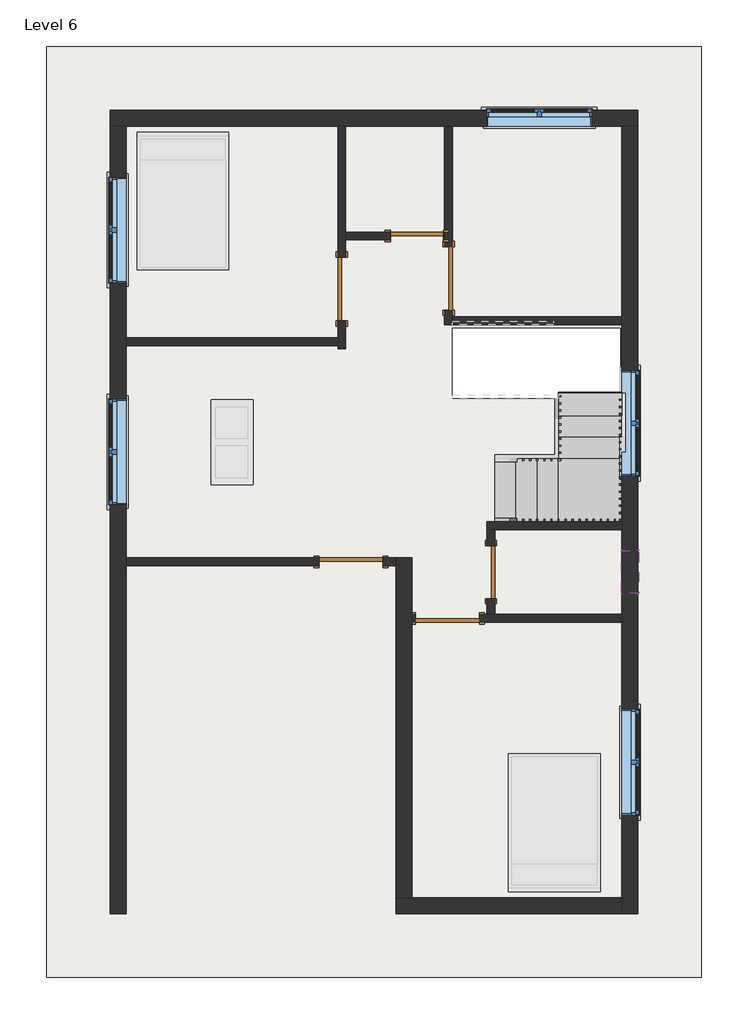
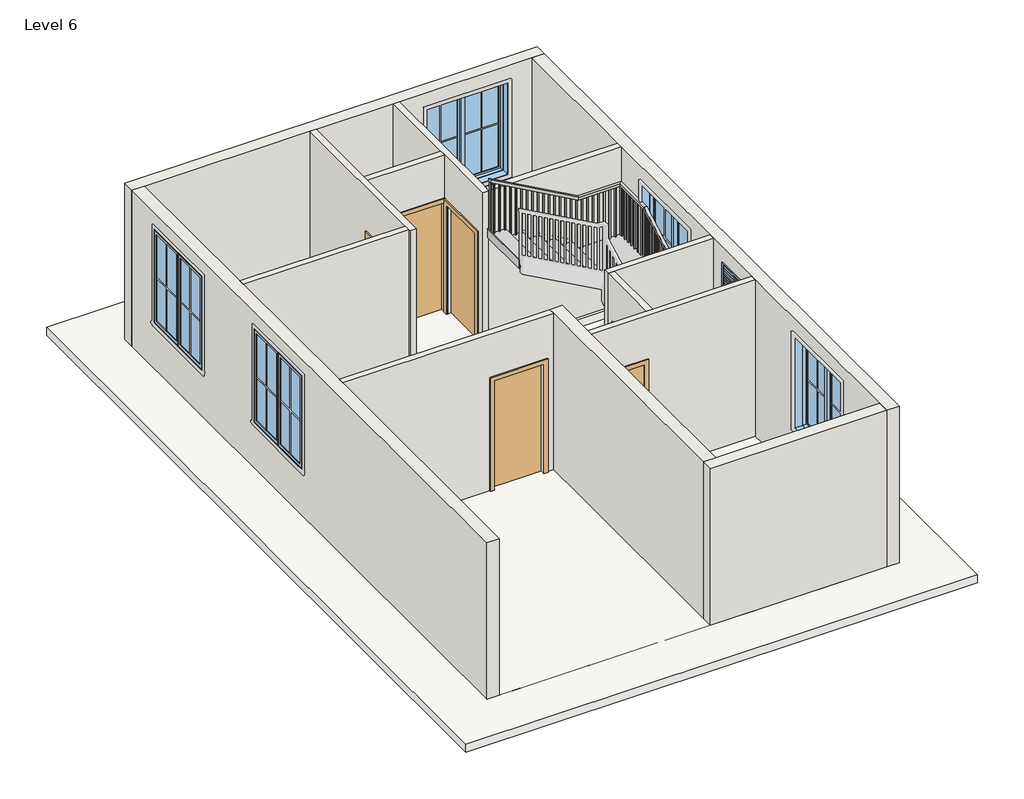
# One storey, part 1 of 2: 14 walls, 6 doors, 6 windows, 1 railing, 1 roof, 1 slab, 1 stair flight.
"""IFC4 building model written with IfcOpenShell, lengths in millimetres."""

from ifc_helpers import new_model, si_unit, frame, origin, place, context, project, spatial, polyline, outline, extrude, faceted_brep, transform, mapped, element, save
from components import door_214872d5, door_78caadf7, single_flush_door_3_e5f9f3c4, single_flush_door_3_305aa2a5, stair_flight_371ece70, window_casement_double_win_5_f93960c7, window_f2d8fef0

model = new_model("IFC4")

# Units and contexts
model_context = context("Model", 3, world=origin())
ifc_project = project(units=[si_unit("LENGTHUNIT", "METRE", prefix="MILLI")], contexts=[model_context])

# Site, building, storey
site = spatial("IfcSite", under=ifc_project)
building = spatial("IfcBuilding", under=site)
storey = spatial("IfcBuildingStorey", under=building, Name="Level 6", Elevation=12801.6)

# Doors
placement = place(None, origin())
door_shape = door_214872d5(model_context)
element("IfcDoor", 1, ObjectType="Single-Flush : DOOR 2'6\"", at=placement, inside=storey, context=model_context, shape_type="MappedRepresentation", body=[
    mapped(door_shape, transform((-185.4325206, 3926.3629493, 12801.6), x_axis=(1.0, 0.0, 0.0), y_axis=(0.0, 1.0, 0.0), z_axis=(0.0, 0.0, 1.0))),
])
door_2_shape = door_78caadf7(model_context)
element("IfcDoor", 2, ObjectType="Single-Flush : DOOR 2'6\"", at=placement, inside=storey, context=model_context, shape_type="MappedRepresentation", body=[
    mapped(door_2_shape, transform((881.3674794, -905.9870507, 12801.6), x_axis=(0.0, 1.0, 0.0), y_axis=(-1.0, 0.0, 0.0), z_axis=(0.0, 0.0, 1.0))),
])
single_flush_door_3_shape = single_flush_door_3_e5f9f3c4(model_context)
element("IfcDoor", 3, ObjectType="Single-Flush : DOOR 3'", at=placement, inside=storey, context=model_context, shape_type="MappedRepresentation", body=[
    mapped(single_flush_door_3_shape, transform((271.7674794, 3316.7629493, 12801.6), x_axis=(0.0, -1.0, 0.0), y_axis=(1.0, 0.0, 0.0), z_axis=(0.0, 0.0, 1.0))),
])
element("IfcDoor", 4, ObjectType="Single-Flush : DOOR 3'", at=placement, inside=storey, context=model_context, shape_type="MappedRepresentation", body=[
    mapped(single_flush_door_3_shape, transform((255.8924794, -1572.7370507, 12801.6), x_axis=(-1.0, 0.0, 0.0), y_axis=(0.0, -1.0, 0.0), z_axis=(0.0, 0.0, 1.0))),
])
single_flush_door_3_2_shape = single_flush_door_3_305aa2a5(model_context)
element("IfcDoor", 5, ObjectType="Single-Flush : DOOR 3'", at=placement, inside=storey, context=model_context, shape_type="MappedRepresentation", body=[
    mapped(single_flush_door_3_2_shape, transform((-1264.9325206, 3164.3629493, 12801.6), x_axis=(0.0, -1.0, 0.0), y_axis=(1.0, 0.0, 0.0), z_axis=(0.0, 0.0, 1.0))),
])
element("IfcDoor", 6, ObjectType="Single-Flush : DOOR 3'6\"", at=placement, inside=storey, context=model_context, shape_type="MappedRepresentation", body=[
    mapped(single_flush_door_3_shape, transform((-1131.5825206, -759.9370507, 12801.6), x_axis=(1.0, 0.0, 0.0), y_axis=(0.0, 1.0, 0.0), z_axis=(0.0, 0.0, 1.0))),
])

# Railing
element("IfcRailing", 7, ObjectType="Handrail - Rectangular", at=placement, inside=storey, context=model_context, shape_type="SolidModel", body=[
    faceted_brep([(938.5174794, -131.2870507, 13885.3333333), (938.5174794, -131.2870507, 13827.220221), (938.5174794, -182.0870507, 13827.220221), (938.5174794, -182.0870507, 13885.3333333), (2005.3174794, -131.2870507, 14478.0), (2018.4810817, -131.2870507, 14427.2), (2018.4810817, -182.0870507, 14427.2), (2005.3174794, -182.0870507, 14478.0), (2716.5174794, -131.2870507, 14478.0), (2716.5174794, -131.2870507, 14427.2), (2767.3174794, -182.0870507, 14427.2), (2767.3174794, -182.0870507, 14478.0), (2716.5174794, 579.9129493, 14478.0), (2716.5174794, 593.0765516, 14427.2), (2767.3174794, 593.0765516, 14427.2), (2767.3174794, 579.9129493, 14478.0), (2716.5174794, 1843.5629493, 15180.0277778), (2716.5174794, 1856.7265516, 15129.2277778), (2767.3174794, 1856.7265516, 15129.2277778), (2767.3174794, 1843.5629493, 15180.0277778), (2716.5174794, 2599.2129493, 15180.0277778), (2716.5174794, 2599.2129493, 15129.2277778), (2767.3174794, 2650.0129493, 15129.2277778), (2767.3174794, 2650.0129493, 15180.0277778), (1960.8674794, 2599.2129493, 15180.0277778), (1947.7038772, 2599.2129493, 15129.2277778), (1947.7038772, 2650.0129493, 15129.2277778), (1960.8674794, 2650.0129493, 15180.0277778), (328.9174794, 2599.2129493, 16086.6666667), (328.9174794, 2650.0129493, 16086.6666667), (328.9174794, 2650.0129493, 16028.5535543), (328.9174794, 2599.2129493, 16028.5535543)], [[[0, 1, 2, 3]], [[1, 0, 4, 5]], [[2, 1, 5, 6]], [[3, 2, 6, 7]], [[0, 3, 7, 4]], [[5, 4, 8, 9]], [[6, 5, 9, 10]], [[7, 6, 10, 11]], [[4, 7, 11, 8]], [[9, 8, 12, 13]], [[10, 9, 13, 14]], [[11, 10, 14, 15]], [[8, 11, 15, 12]], [[13, 12, 16, 17]], [[14, 13, 17, 18]], [[15, 14, 18, 19]], [[12, 15, 19, 16]], [[17, 16, 20, 21]], [[18, 17, 21, 22]], [[19, 18, 22, 23]], [[16, 19, 23, 20]], [[21, 20, 24, 25]], [[22, 21, 25, 26]], [[23, 22, 26, 27]], [[20, 23, 27, 24]], [[28, 29, 30, 31]], [[25, 24, 28, 31]], [[26, 25, 31, 30]], [[27, 26, 30, 29]], [[24, 27, 29, 28]]]),
    extrude(outline(polyline([(15980.9285543, 414.6424794), (15991.5118876, 395.5924794), (15002.9333333, 395.5924794), (15002.9333333, 414.6424794), (15980.9285543, 414.6424794)])), frame((0.0, 2615.0879493, 0.0), z_axis=(0.0, 1.0, 0.0), x_axis=(0.0, 0.0, 1.0)), (0.0, 0.0, 1.0), 19.05),
    extrude(outline(polyline([(15924.4841099, 516.2424794), (15935.0674432, 497.1924794), (15002.9333333, 497.1924794), (15002.9333333, 516.2424794), (15924.4841099, 516.2424794)])), frame((0.0, 2615.0879493, 0.0), z_axis=(0.0, 1.0, 0.0), x_axis=(0.0, 0.0, 1.0)), (0.0, 0.0, 1.0), 19.05),
    extrude(outline(polyline([(15868.0396654, 617.8424794), (15878.6229988, 598.7924794), (15002.9333333, 598.7924794), (15002.9333333, 617.8424794), (15868.0396654, 617.8424794)])), frame((0.0, 2615.0879493, 0.0), z_axis=(0.0, 1.0, 0.0), x_axis=(0.0, 0.0, 1.0)), (0.0, 0.0, 1.0), 19.05),
    extrude(outline(polyline([(15811.595221, 719.4424794), (15822.1785543, 700.3924794), (14833.6, 700.3924794), (14833.6, 719.4424794), (15811.595221, 719.4424794)])), frame((0.0, 2615.0879493, 0.0), z_axis=(0.0, 1.0, 0.0), x_axis=(0.0, 0.0, 1.0)), (0.0, 0.0, 1.0), 19.05),
    extrude(outline(polyline([(15755.1507765, 821.0424794), (15765.7341099, 801.9924794), (14833.6, 801.9924794), (14833.6, 821.0424794), (15755.1507765, 821.0424794)])), frame((0.0, 2615.0879493, 0.0), z_axis=(0.0, 1.0, 0.0), x_axis=(0.0, 0.0, 1.0)), (0.0, 0.0, 1.0), 19.05),
    extrude(outline(polyline([(15698.7063321, 922.6424794), (15709.2896654, 903.5924794), (14833.6, 903.5924794), (14833.6, 922.6424794), (15698.7063321, 922.6424794)])), frame((0.0, 2615.0879493, 0.0), z_axis=(0.0, 1.0, 0.0), x_axis=(0.0, 0.0, 1.0)), (0.0, 0.0, 1.0), 19.05),
    extrude(outline(polyline([(15642.2618876, 1024.2424794), (15652.845221, 1005.1924794), (14664.2666667, 1005.1924794), (14664.2666667, 1024.2424794), (15642.2618876, 1024.2424794)])), frame((0.0, 2615.0879493, 0.0), z_axis=(0.0, 1.0, 0.0), x_axis=(0.0, 0.0, 1.0)), (0.0, 0.0, 1.0), 19.05),
    extrude(outline(polyline([(15585.8174432, 1125.8424794), (15596.4007765, 1106.7924794), (14664.2666667, 1106.7924794), (14664.2666667, 1125.8424794), (15585.8174432, 1125.8424794)])), frame((0.0, 2615.0879493, 0.0), z_axis=(0.0, 1.0, 0.0), x_axis=(0.0, 0.0, 1.0)), (0.0, 0.0, 1.0), 19.05),
    extrude(outline(polyline([(15529.3729988, 1227.4424794), (15539.9563321, 1208.3924794), (14664.2666667, 1208.3924794), (14664.2666667, 1227.4424794), (15529.3729988, 1227.4424794)])), frame((0.0, 2615.0879493, 0.0), z_axis=(0.0, 1.0, 0.0), x_axis=(0.0, 0.0, 1.0)), (0.0, 0.0, 1.0), 19.05),
    extrude(outline(polyline([(15472.9285543, 1329.0424794), (15483.5118876, 1309.9924794), (14494.9333333, 1309.9924794), (14494.9333333, 1329.0424794), (15472.9285543, 1329.0424794)])), frame((0.0, 2615.0879493, 0.0), z_axis=(0.0, 1.0, 0.0), x_axis=(0.0, 0.0, 1.0)), (0.0, 0.0, 1.0), 19.05),
    extrude(outline(polyline([(15416.4841099, 1430.6424794), (15427.0674432, 1411.5924794), (14494.9333333, 1411.5924794), (14494.9333333, 1430.6424794), (15416.4841099, 1430.6424794)])), frame((0.0, 2615.0879493, 0.0), z_axis=(0.0, 1.0, 0.0), x_axis=(0.0, 0.0, 1.0)), (0.0, 0.0, 1.0), 19.05),
    extrude(outline(polyline([(15360.0396654, 1532.2424794), (15370.6229988, 1513.1924794), (14494.9333333, 1513.1924794), (14494.9333333, 1532.2424794), (15360.0396654, 1532.2424794)])), frame((0.0, 2615.0879493, 0.0), z_axis=(0.0, 1.0, 0.0), x_axis=(0.0, 0.0, 1.0)), (0.0, 0.0, 1.0), 19.05),
    extrude(outline(polyline([(15303.595221, 1633.8424794), (15314.1785543, 1614.7924794), (14325.6, 1614.7924794), (14325.6, 1633.8424794), (15303.595221, 1633.8424794)])), frame((0.0, 2615.0879493, 0.0), z_axis=(0.0, 1.0, 0.0), x_axis=(0.0, 0.0, 1.0)), (0.0, 0.0, 1.0), 19.05),
    extrude(outline(polyline([(15247.1507765, 1735.4424794), (15257.7341099, 1716.3924794), (14325.6, 1716.3924794), (14325.6, 1735.4424794), (15247.1507765, 1735.4424794)])), frame((0.0, 2615.0879493, 0.0), z_axis=(0.0, 1.0, 0.0), x_axis=(0.0, 0.0, 1.0)), (0.0, 0.0, 1.0), 19.05),
    extrude(outline(polyline([(15190.7063321, 1837.0424794), (15201.2896654, 1817.9924794), (14325.6, 1817.9924794), (14325.6, 1837.0424794), (15190.7063321, 1837.0424794)])), frame((0.0, 2615.0879493, 0.0), z_axis=(0.0, 1.0, 0.0), x_axis=(0.0, 0.0, 1.0)), (0.0, 0.0, 1.0), 19.05),
    extrude(outline(polyline([(15134.2618876, 1938.6424794), (15144.845221, 1919.5924794), (14156.2666667, 1919.5924794), (14156.2666667, 1938.6424794), (15134.2618876, 1938.6424794)])), frame((0.0, 2615.0879493, 0.0), z_axis=(0.0, 1.0, 0.0), x_axis=(0.0, 0.0, 1.0)), (0.0, 0.0, 1.0), 19.05),
    extrude(outline(polyline([(2040.2424794, 2634.1379493), (2040.2424794, 2615.0879493), (2021.1924794, 2615.0879493), (2021.1924794, 2634.1379493), (2040.2424794, 2634.1379493)])), frame((0.0, 0.0, 14156.2666667), z_axis=(0.0, 0.0, 1.0), x_axis=(1.0, 0.0, 0.0)), (0.0, 0.0, 1.0), 972.9611111),
    extrude(outline(polyline([(2141.8424794, 2634.1379493), (2141.8424794, 2615.0879493), (2122.7924794, 2615.0879493), (2122.7924794, 2634.1379493), (2141.8424794, 2634.1379493)])), frame((0.0, 0.0, 14156.2666667), z_axis=(0.0, 0.0, 1.0), x_axis=(1.0, 0.0, 0.0)), (0.0, 0.0, 1.0), 972.9611111),
    extrude(outline(polyline([(2243.4424794, 2634.1379493), (2243.4424794, 2615.0879493), (2224.3924794, 2615.0879493), (2224.3924794, 2634.1379493), (2243.4424794, 2634.1379493)])), frame((0.0, 0.0, 14156.2666667), z_axis=(0.0, 0.0, 1.0), x_axis=(1.0, 0.0, 0.0)), (0.0, 0.0, 1.0), 972.9611111),
    extrude(outline(polyline([(2345.0424794, 2634.1379493), (2345.0424794, 2615.0879493), (2325.9924794, 2615.0879493), (2325.9924794, 2634.1379493), (2345.0424794, 2634.1379493)])), frame((0.0, 0.0, 14156.2666667), z_axis=(0.0, 0.0, 1.0), x_axis=(1.0, 0.0, 0.0)), (0.0, 0.0, 1.0), 972.9611111),
    extrude(outline(polyline([(2446.6424794, 2634.1379493), (2446.6424794, 2615.0879493), (2427.5924794, 2615.0879493), (2427.5924794, 2634.1379493), (2446.6424794, 2634.1379493)])), frame((0.0, 0.0, 14156.2666667), z_axis=(0.0, 0.0, 1.0), x_axis=(1.0, 0.0, 0.0)), (0.0, 0.0, 1.0), 972.9611111),
    extrude(outline(polyline([(2548.2424794, 2634.1379493), (2548.2424794, 2615.0879493), (2529.1924794, 2615.0879493), (2529.1924794, 2634.1379493), (2548.2424794, 2634.1379493)])), frame((0.0, 0.0, 14156.2666667), z_axis=(0.0, 0.0, 1.0), x_axis=(1.0, 0.0, 0.0)), (0.0, 0.0, 1.0), 972.9611111),
    extrude(outline(polyline([(2649.8424794, 2634.1379493), (2649.8424794, 2615.0879493), (2630.7924794, 2615.0879493), (2630.7924794, 2634.1379493), (2649.8424794, 2634.1379493)])), frame((0.0, 0.0, 14156.2666667), z_axis=(0.0, 0.0, 1.0), x_axis=(1.0, 0.0, 0.0)), (0.0, 0.0, 1.0), 972.9611111),
    extrude(outline(polyline([(2751.4424794, 2576.9879493), (2732.3924794, 2576.9879493), (2732.3924794, 2596.0379493), (2751.4424794, 2596.0379493), (2751.4424794, 2576.9879493)])), frame((0.0, 0.0, 14156.2666667), z_axis=(0.0, 0.0, 1.0), x_axis=(1.0, 0.0, 0.0)), (0.0, 0.0, 1.0), 972.9611111),
    extrude(outline(polyline([(2751.4424794, 2475.3879493), (2732.3924794, 2475.3879493), (2732.3924794, 2494.4379493), (2751.4424794, 2494.4379493), (2751.4424794, 2475.3879493)])), frame((0.0, 0.0, 14156.2666667), z_axis=(0.0, 0.0, 1.0), x_axis=(1.0, 0.0, 0.0)), (0.0, 0.0, 1.0), 972.9611111),
    extrude(outline(polyline([(2751.4424794, 2373.7879493), (2732.3924794, 2373.7879493), (2732.3924794, 2392.8379493), (2751.4424794, 2392.8379493), (2751.4424794, 2373.7879493)])), frame((0.0, 0.0, 14156.2666667), z_axis=(0.0, 0.0, 1.0), x_axis=(1.0, 0.0, 0.0)), (0.0, 0.0, 1.0), 972.9611111),
    extrude(outline(polyline([(2751.4424794, 2272.1879493), (2732.3924794, 2272.1879493), (2732.3924794, 2291.2379493), (2751.4424794, 2291.2379493), (2751.4424794, 2272.1879493)])), frame((0.0, 0.0, 14156.2666667), z_axis=(0.0, 0.0, 1.0), x_axis=(1.0, 0.0, 0.0)), (0.0, 0.0, 1.0), 972.9611111),
    extrude(outline(polyline([(2751.4424794, 2170.5879493), (2732.3924794, 2170.5879493), (2732.3924794, 2189.6379493), (2751.4424794, 2189.6379493), (2751.4424794, 2170.5879493)])), frame((0.0, 0.0, 14156.2666667), z_axis=(0.0, 0.0, 1.0), x_axis=(1.0, 0.0, 0.0)), (0.0, 0.0, 1.0), 972.9611111),
    extrude(outline(polyline([(2751.4424794, 2068.9879493), (2732.3924794, 2068.9879493), (2732.3924794, 2088.0379493), (2751.4424794, 2088.0379493), (2751.4424794, 2068.9879493)])), frame((0.0, 0.0, 14156.2666667), z_axis=(0.0, 0.0, 1.0), x_axis=(1.0, 0.0, 0.0)), (0.0, 0.0, 1.0), 972.9611111),
    extrude(outline(polyline([(2751.4424794, 1967.3879493), (2732.3924794, 1967.3879493), (2732.3924794, 1986.4379493), (2751.4424794, 1986.4379493), (2751.4424794, 1967.3879493)])), frame((0.0, 0.0, 14156.2666667), z_axis=(0.0, 0.0, 1.0), x_axis=(1.0, 0.0, 0.0)), (0.0, 0.0, 1.0), 972.9611111),
    extrude(outline(polyline([(2751.4424794, 1865.7879493), (2732.3924794, 1865.7879493), (2732.3924794, 1884.8379493), (2751.4424794, 1884.8379493), (2751.4424794, 1865.7879493)])), frame((0.0, 0.0, 14156.2666667), z_axis=(0.0, 0.0, 1.0), x_axis=(1.0, 0.0, 0.0)), (0.0, 0.0, 1.0), 972.9611111),
    extrude(outline(polyline([(1764.1879493, 15077.8174432), (1783.2379493, 15088.4007765), (1783.2379493, 14156.2666667), (1764.1879493, 14156.2666667), (1764.1879493, 15077.8174432)])), frame((2732.3924794, 0.0, 0.0), z_axis=(1.0, 0.0, 0.0), x_axis=(0.0, 1.0, 0.0)), (0.0, 0.0, 1.0), 19.05),
    extrude(outline(polyline([(1662.5879493, 15021.3729988), (1681.6379493, 15031.9563321), (1681.6379493, 14156.2666667), (1662.5879493, 14156.2666667), (1662.5879493, 15021.3729988)])), frame((2732.3924794, 0.0, 0.0), z_axis=(1.0, 0.0, 0.0), x_axis=(0.0, 1.0, 0.0)), (0.0, 0.0, 1.0), 19.05),
    extrude(outline(polyline([(1560.9879493, 14964.9285543), (1580.0379493, 14975.5118876), (1580.0379493, 13986.9333333), (1560.9879493, 13986.9333333), (1560.9879493, 14964.9285543)])), frame((2732.3924794, 0.0, 0.0), z_axis=(1.0, 0.0, 0.0), x_axis=(0.0, 1.0, 0.0)), (0.0, 0.0, 1.0), 19.05),
    extrude(outline(polyline([(1459.3879493, 14908.4841099), (1478.4379493, 14919.0674432), (1478.4379493, 13986.9333333), (1459.3879493, 13986.9333333), (1459.3879493, 14908.4841099)])), frame((2732.3924794, 0.0, 0.0), z_axis=(1.0, 0.0, 0.0), x_axis=(0.0, 1.0, 0.0)), (0.0, 0.0, 1.0), 19.05),
    extrude(outline(polyline([(1357.7879493, 14852.0396654), (1376.8379493, 14862.6229988), (1376.8379493, 13986.9333333), (1357.7879493, 13986.9333333), (1357.7879493, 14852.0396654)])), frame((2732.3924794, 0.0, 0.0), z_axis=(1.0, 0.0, 0.0), x_axis=(0.0, 1.0, 0.0)), (0.0, 0.0, 1.0), 19.05),
    extrude(outline(polyline([(1256.1879493, 14795.595221), (1275.2379493, 14806.1785543), (1275.2379493, 13817.6), (1256.1879493, 13817.6), (1256.1879493, 14795.595221)])), frame((2732.3924794, 0.0, 0.0), z_axis=(1.0, 0.0, 0.0), x_axis=(0.0, 1.0, 0.0)), (0.0, 0.0, 1.0), 19.05),
    extrude(outline(polyline([(1154.5879493, 14739.1507765), (1173.6379493, 14749.7341099), (1173.6379493, 13817.6), (1154.5879493, 13817.6), (1154.5879493, 14739.1507765)])), frame((2732.3924794, 0.0, 0.0), z_axis=(1.0, 0.0, 0.0), x_axis=(0.0, 1.0, 0.0)), (0.0, 0.0, 1.0), 19.05),
    extrude(outline(polyline([(1052.9879493, 14682.7063321), (1072.0379493, 14693.2896654), (1072.0379493, 13817.6), (1052.9879493, 13817.6), (1052.9879493, 14682.7063321)])), frame((2732.3924794, 0.0, 0.0), z_axis=(1.0, 0.0, 0.0), x_axis=(0.0, 1.0, 0.0)), (0.0, 0.0, 1.0), 19.05),
    extrude(outline(polyline([(951.3879493, 14626.2618876), (970.4379493, 14636.845221), (970.4379493, 13648.2666667), (951.3879493, 13648.2666667), (951.3879493, 14626.2618876)])), frame((2732.3924794, 0.0, 0.0), z_axis=(1.0, 0.0, 0.0), x_axis=(0.0, 1.0, 0.0)), (0.0, 0.0, 1.0), 19.05),
    extrude(outline(polyline([(849.7879493, 14569.8174432), (868.8379493, 14580.4007765), (868.8379493, 13648.2666667), (849.7879493, 13648.2666667), (849.7879493, 14569.8174432)])), frame((2732.3924794, 0.0, 0.0), z_axis=(1.0, 0.0, 0.0), x_axis=(0.0, 1.0, 0.0)), (0.0, 0.0, 1.0), 19.05),
    extrude(outline(polyline([(748.1879493, 14513.3729988), (767.2379493, 14523.9563321), (767.2379493, 13648.2666667), (748.1879493, 13648.2666667), (748.1879493, 14513.3729988)])), frame((2732.3924794, 0.0, 0.0), z_axis=(1.0, 0.0, 0.0), x_axis=(0.0, 1.0, 0.0)), (0.0, 0.0, 1.0), 19.05),
    extrude(outline(polyline([(646.5879493, 14456.9285543), (665.6379493, 14467.5118876), (665.6379493, 13478.9333333), (646.5879493, 13478.9333333), (646.5879493, 14456.9285543)])), frame((2732.3924794, 0.0, 0.0), z_axis=(1.0, 0.0, 0.0), x_axis=(0.0, 1.0, 0.0)), (0.0, 0.0, 1.0), 19.05),
    extrude(outline(polyline([(2751.4424794, 544.9879493), (2732.3924794, 544.9879493), (2732.3924794, 564.0379493), (2751.4424794, 564.0379493), (2751.4424794, 544.9879493)])), frame((0.0, 0.0, 13478.9333333), z_axis=(0.0, 0.0, 1.0), x_axis=(1.0, 0.0, 0.0)), (0.0, 0.0, 1.0), 948.2666667),
    extrude(outline(polyline([(2751.4424794, 443.3879493), (2732.3924794, 443.3879493), (2732.3924794, 462.4379493), (2751.4424794, 462.4379493), (2751.4424794, 443.3879493)])), frame((0.0, 0.0, 13478.9333333), z_axis=(0.0, 0.0, 1.0), x_axis=(1.0, 0.0, 0.0)), (0.0, 0.0, 1.0), 948.2666667),
    extrude(outline(polyline([(2751.4424794, 341.7879493), (2732.3924794, 341.7879493), (2732.3924794, 360.8379493), (2751.4424794, 360.8379493), (2751.4424794, 341.7879493)])), frame((0.0, 0.0, 13478.9333333), z_axis=(0.0, 0.0, 1.0), x_axis=(1.0, 0.0, 0.0)), (0.0, 0.0, 1.0), 948.2666667),
    extrude(outline(polyline([(2751.4424794, 240.1879493), (2732.3924794, 240.1879493), (2732.3924794, 259.2379493), (2751.4424794, 259.2379493), (2751.4424794, 240.1879493)])), frame((0.0, 0.0, 13478.9333333), z_axis=(0.0, 0.0, 1.0), x_axis=(1.0, 0.0, 0.0)), (0.0, 0.0, 1.0), 948.2666667),
    extrude(outline(polyline([(2751.4424794, 138.5879493), (2732.3924794, 138.5879493), (2732.3924794, 157.6379493), (2751.4424794, 157.6379493), (2751.4424794, 138.5879493)])), frame((0.0, 0.0, 13478.9333333), z_axis=(0.0, 0.0, 1.0), x_axis=(1.0, 0.0, 0.0)), (0.0, 0.0, 1.0), 948.2666667),
    extrude(outline(polyline([(2751.4424794, 36.9879493), (2732.3924794, 36.9879493), (2732.3924794, 56.0379493), (2751.4424794, 56.0379493), (2751.4424794, 36.9879493)])), frame((0.0, 0.0, 13478.9333333), z_axis=(0.0, 0.0, 1.0), x_axis=(1.0, 0.0, 0.0)), (0.0, 0.0, 1.0), 948.2666667),
    extrude(outline(polyline([(2751.4424794, -64.6120507), (2732.3924794, -64.6120507), (2732.3924794, -45.5620507), (2751.4424794, -45.5620507), (2751.4424794, -64.6120507)])), frame((0.0, 0.0, 13478.9333333), z_axis=(0.0, 0.0, 1.0), x_axis=(1.0, 0.0, 0.0)), (0.0, 0.0, 1.0), 948.2666667),
    extrude(outline(polyline([(2656.1924794, -166.2120507), (2656.1924794, -147.1620507), (2675.2424794, -147.1620507), (2675.2424794, -166.2120507), (2656.1924794, -166.2120507)])), frame((0.0, 0.0, 13478.9333333), z_axis=(0.0, 0.0, 1.0), x_axis=(1.0, 0.0, 0.0)), (0.0, 0.0, 1.0), 948.2666667),
    extrude(outline(polyline([(2554.5924794, -166.2120507), (2554.5924794, -147.1620507), (2573.6424794, -147.1620507), (2573.6424794, -166.2120507), (2554.5924794, -166.2120507)])), frame((0.0, 0.0, 13478.9333333), z_axis=(0.0, 0.0, 1.0), x_axis=(1.0, 0.0, 0.0)), (0.0, 0.0, 1.0), 948.2666667),
    extrude(outline(polyline([(2452.9924794, -166.2120507), (2452.9924794, -147.1620507), (2472.0424794, -147.1620507), (2472.0424794, -166.2120507), (2452.9924794, -166.2120507)])), frame((0.0, 0.0, 13478.9333333), z_axis=(0.0, 0.0, 1.0), x_axis=(1.0, 0.0, 0.0)), (0.0, 0.0, 1.0), 948.2666667),
    extrude(outline(polyline([(2351.3924794, -166.2120507), (2351.3924794, -147.1620507), (2370.4424794, -147.1620507), (2370.4424794, -166.2120507), (2351.3924794, -166.2120507)])), frame((0.0, 0.0, 13478.9333333), z_axis=(0.0, 0.0, 1.0), x_axis=(1.0, 0.0, 0.0)), (0.0, 0.0, 1.0), 948.2666667),
    extrude(outline(polyline([(2249.7924794, -166.2120507), (2249.7924794, -147.1620507), (2268.8424794, -147.1620507), (2268.8424794, -166.2120507), (2249.7924794, -166.2120507)])), frame((0.0, 0.0, 13478.9333333), z_axis=(0.0, 0.0, 1.0), x_axis=(1.0, 0.0, 0.0)), (0.0, 0.0, 1.0), 948.2666667),
    extrude(outline(polyline([(2148.1924794, -166.2120507), (2148.1924794, -147.1620507), (2167.2424794, -147.1620507), (2167.2424794, -166.2120507), (2148.1924794, -166.2120507)])), frame((0.0, 0.0, 13478.9333333), z_axis=(0.0, 0.0, 1.0), x_axis=(1.0, 0.0, 0.0)), (0.0, 0.0, 1.0), 948.2666667),
    extrude(outline(polyline([(2046.5924794, -166.2120507), (2046.5924794, -147.1620507), (2065.6424794, -147.1620507), (2065.6424794, -166.2120507), (2046.5924794, -166.2120507)])), frame((0.0, 0.0, 13478.9333333), z_axis=(0.0, 0.0, 1.0), x_axis=(1.0, 0.0, 0.0)), (0.0, 0.0, 1.0), 948.2666667),
    extrude(outline(polyline([(14396.9563321, 1964.0424794), (14386.3729988, 1944.9924794), (13478.9333333, 1944.9924794), (13478.9333333, 1964.0424794), (14396.9563321, 1964.0424794)])), frame((0.0, -166.2120507, 0.0), z_axis=(0.0, 1.0, 0.0), x_axis=(0.0, 0.0, 1.0)), (0.0, 0.0, 1.0), 19.05),
    extrude(outline(polyline([(14340.5118876, 1862.4424794), (14329.9285543, 1843.3924794), (13478.9333333, 1843.3924794), (13478.9333333, 1862.4424794), (14340.5118876, 1862.4424794)])), frame((0.0, -166.2120507, 0.0), z_axis=(0.0, 1.0, 0.0), x_axis=(0.0, 0.0, 1.0)), (0.0, 0.0, 1.0), 19.05),
    extrude(outline(polyline([(14284.0674432, 1760.8424794), (14273.4841099, 1741.7924794), (13309.6, 1741.7924794), (13309.6, 1760.8424794), (14284.0674432, 1760.8424794)])), frame((0.0, -166.2120507, 0.0), z_axis=(0.0, 1.0, 0.0), x_axis=(0.0, 0.0, 1.0)), (0.0, 0.0, 1.0), 19.05),
    extrude(outline(polyline([(14227.6229988, 1659.2424794), (14217.0396654, 1640.1924794), (13309.6, 1640.1924794), (13309.6, 1659.2424794), (14227.6229988, 1659.2424794)])), frame((0.0, -166.2120507, 0.0), z_axis=(0.0, 1.0, 0.0), x_axis=(0.0, 0.0, 1.0)), (0.0, 0.0, 1.0), 19.05),
    extrude(outline(polyline([(14171.1785543, 1557.6424794), (14160.595221, 1538.5924794), (13309.6, 1538.5924794), (13309.6, 1557.6424794), (14171.1785543, 1557.6424794)])), frame((0.0, -166.2120507, 0.0), z_axis=(0.0, 1.0, 0.0), x_axis=(0.0, 0.0, 1.0)), (0.0, 0.0, 1.0), 19.05),
    extrude(outline(polyline([(14114.7341099, 1456.0424794), (14104.1507765, 1436.9924794), (13140.2666667, 1436.9924794), (13140.2666667, 1456.0424794), (14114.7341099, 1456.0424794)])), frame((0.0, -166.2120507, 0.0), z_axis=(0.0, 1.0, 0.0), x_axis=(0.0, 0.0, 1.0)), (0.0, 0.0, 1.0), 19.05),
    extrude(outline(polyline([(14058.2896654, 1354.4424794), (14047.7063321, 1335.3924794), (13140.2666667, 1335.3924794), (13140.2666667, 1354.4424794), (14058.2896654, 1354.4424794)])), frame((0.0, -166.2120507, 0.0), z_axis=(0.0, 1.0, 0.0), x_axis=(0.0, 0.0, 1.0)), (0.0, 0.0, 1.0), 19.05),
    extrude(outline(polyline([(14001.845221, 1252.8424794), (13991.2618876, 1233.7924794), (13140.2666667, 1233.7924794), (13140.2666667, 1252.8424794), (14001.845221, 1252.8424794)])), frame((0.0, -166.2120507, 0.0), z_axis=(0.0, 1.0, 0.0), x_axis=(0.0, 0.0, 1.0)), (0.0, 0.0, 1.0), 19.05),
    extrude(outline(polyline([(13945.4007765, 1151.2424794), (13934.8174432, 1132.1924794), (12970.9333333, 1132.1924794), (12970.9333333, 1151.2424794), (13945.4007765, 1151.2424794)])), frame((0.0, -166.2120507, 0.0), z_axis=(0.0, 1.0, 0.0), x_axis=(0.0, 0.0, 1.0)), (0.0, 0.0, 1.0), 19.05),
    extrude(outline(polyline([(13888.9563321, 1049.6424794), (13878.3729988, 1030.5924794), (12970.9333333, 1030.5924794), (12970.9333333, 1049.6424794), (13888.9563321, 1049.6424794)])), frame((0.0, -166.2120507, 0.0), z_axis=(0.0, 1.0, 0.0), x_axis=(0.0, 0.0, 1.0)), (0.0, 0.0, 1.0), 19.05),
    extrude(outline(polyline([(2751.4424794, 2615.0879493), (2732.3924794, 2615.0879493), (2732.3924794, 2634.1379493), (2751.4424794, 2634.1379493), (2751.4424794, 2615.0879493)])), frame((0.0, 0.0, 14156.2666667), z_axis=(0.0, 0.0, 1.0), x_axis=(1.0, 0.0, 0.0)), (0.0, 0.0, 1.0), 972.9611111),
    extrude(outline(polyline([(2732.3924794, -166.2120507), (2732.3924794, -147.1620507), (2751.4424794, -147.1620507), (2751.4424794, -166.2120507), (2732.3924794, -166.2120507)])), frame((0.0, 0.0, 13478.9333333), z_axis=(0.0, 0.0, 1.0), x_axis=(1.0, 0.0, 0.0)), (0.0, 0.0, 1.0), 948.2666667),
    extrude(outline(polyline([(16017.970221, 347.9674794), (16028.5535543, 328.9174794), (15002.9333333, 328.9174794), (15002.9333333, 347.9674794), (16017.970221, 347.9674794)])), frame((0.0, 2615.0879493, 0.0), z_axis=(0.0, 1.0, 0.0), x_axis=(0.0, 0.0, 1.0)), (0.0, 0.0, 1.0), 19.05),
    extrude(outline(polyline([(13837.8035543, 957.5674794), (13827.220221, 938.5174794), (12970.9333333, 938.5174794), (12970.9333333, 957.5674794), (13837.8035543, 957.5674794)])), frame((0.0, -166.2120507, 0.0), z_axis=(0.0, 1.0, 0.0), x_axis=(0.0, 0.0, 1.0)), (0.0, 0.0, 1.0), 19.05),
])

# Roof
element("IfcRoof", 8, ObjectType="ROOF 6\"", at=placement, inside=storey, context=model_context, shape_type="SweptSolid", body=[
    extrude(outline(polyline([(-5513.0825206, 6650.5129493), (3910.3174794, 6650.5129493), (3910.3174794, -6735.2870507), (-5513.0825206, -6735.2870507), (-5513.0825206, 6650.5129493)]), holes=[polyline([(2741.9174794, -156.6870507), (2741.9174794, 2599.2129493), (328.9174794, 2599.2129493), (328.9174794, 1595.9129493), (1802.1174794, 1595.9129493), (1802.1174794, 706.9129493), (1040.1174794, 706.9129493), (1040.1174794, -156.6870507), (2741.9174794, -156.6870507)])]), frame((0.0, 0.0, 12649.2), z_axis=(0.0, 0.0, 1.0), x_axis=(1.0, 0.0, 0.0)), (0.0, 0.0, 1.0), 152.4),
])

# Slab
element("IfcSlab", 9, ObjectType="FLOOR 6\"", at=placement, inside=storey, context=model_context, shape_type="SweptSolid", body=[
    extrude(outline(polyline([(2995.9174794, 5736.1129493), (2995.9174794, -5820.8870507), (-4598.6825206, -5820.8870507), (-4598.6825206, 5736.1129493), (2995.9174794, 5736.1129493)]), holes=[polyline([(2741.9174794, -156.6870507), (2741.9174794, 2599.2129493), (328.9174794, 2599.2129493), (328.9174794, 1595.9129493), (1802.1174794, 1595.9129493), (1802.1174794, 706.9129493), (1040.1174794, 706.9129493), (1040.1174794, -156.6870507), (2741.9174794, -156.6870507)])]), frame((0.0, 0.0, 12649.2), z_axis=(0.0, 0.0, 1.0), x_axis=(1.0, 0.0, 0.0)), (0.0, 0.0, 1.0), 152.4),
])

# Stair flight
stair_flight_shape = stair_flight_371ece70(model_context)
element("IfcStairFlight", 10, ObjectType="2\" Tread 1\" Nosing 1/4\" Riser", at=placement, inside=storey, context=model_context, shape_type="MappedRepresentation", body=[
    mapped(stair_flight_shape, transform((0.0, 0.0, 0.0), x_axis=(1.0, 0.0, 0.0), y_axis=(0.0, 1.0, 0.0), z_axis=(0.0, 0.0, 1.0))),
])

# Walls
element("IfcWall", 11, at=placement, inside=storey, context=model_context, shape_type="Brep", body=[
    faceted_brep([(-1322.0825206, 2707.1629493, 14935.2), (-1322.0825206, 2707.1629493, 12801.6), (-1322.0825206, 2459.5129493, 12801.6), (-1322.0825206, 2345.2129493, 12801.6), (-1322.0825206, 2307.1129493, 12801.6), (-1322.0825206, 2307.1129493, 15849.6), (-1322.0825206, 2345.2129493, 15849.6), (-1322.0825206, 2459.5129493, 15849.6), (-1322.0825206, 5507.5129493, 15849.6), (-1322.0825206, 5507.5129493, 12801.6), (-1322.0825206, 3621.5629493, 12801.6), (-1322.0825206, 3621.5629493, 14935.2), (-1207.7825206, 2307.1129493, 12801.6), (-1207.7825206, 2707.1629493, 12801.6), (-1207.7825206, 2707.1629493, 14935.2), (-1207.7825206, 3621.5629493, 14935.2), (-1207.7825206, 3621.5629493, 12801.6), (-1207.7825206, 3869.2129493, 12801.6), (-1207.7825206, 3983.5129493, 12801.6), (-1207.7825206, 5507.5129493, 12801.6), (-1207.7825206, 5507.5129493, 15849.6), (-1207.7825206, 3983.5129493, 15849.6), (-1207.7825206, 3869.2129493, 15849.6), (-1207.7825206, 2307.1129493, 15849.6)], [[[0, 1, 2, 3, 4, 5, 6, 7, 8, 9, 10, 11]], [[12, 13, 14, 15, 16, 17, 18, 19, 20, 21, 22, 23]], [[10, 9, 19, 18, 17, 16]], [[4, 3, 2, 1, 13, 12]], [[5, 4, 12, 23]], [[9, 8, 20, 19]], [[14, 13, 1, 0]], [[15, 14, 0, 11]], [[16, 15, 11, 10]], [[8, 7, 6, 5, 23, 22, 21, 20]]]),
])
element("IfcWall", 12, at=placement, inside=storey, context=model_context, shape_type="SweptSolid", body=[
    extrude(outline(polyline([(-1322.0825206, 2345.2129493), (-4370.0825206, 2345.2129493), (-4370.0825206, 2459.5129493), (-1322.0825206, 2459.5129493), (-1322.0825206, 2345.2129493)])), frame((0.0, 0.0, 12801.6), z_axis=(0.0, 0.0, 1.0), x_axis=(1.0, 0.0, 0.0)), (0.0, 0.0, 1.0), 3048.0),
])
element("IfcWall", 13, at=placement, inside=storey, context=model_context, shape_type="SweptSolid", body=[
    extrude(outline(polyline([(14935.2, 195.5674794), (12801.6, 195.5674794), (12801.6, 214.6174794), (15849.6, 214.6174794), (15849.6, -1207.7825206), (12801.6, -1207.7825206), (12801.6, -566.4325206), (14935.2, -566.4325206), (14935.2, 195.5674794)])), frame((0.0, 3869.2129493, 0.0), z_axis=(0.0, 1.0, 0.0), x_axis=(0.0, 0.0, 1.0)), (0.0, 0.0, 1.0), 114.3),
])
element("IfcWall", 14, at=placement, inside=storey, context=model_context, shape_type="Brep", body=[
    faceted_brep([(214.6174794, 2859.5629493, 14935.2), (214.6174794, 2859.5629493, 12801.6), (214.6174794, 2650.0129493, 12801.6), (214.6174794, 2650.0129493, 15849.6), (214.6174794, 3869.2129493, 15849.6), (214.6174794, 3983.5129493, 15849.6), (214.6174794, 5507.5129493, 15849.6), (214.6174794, 5507.5129493, 12801.6), (214.6174794, 3983.5129493, 12801.6), (214.6174794, 3869.2129493, 12801.6), (214.6174794, 3773.9629493, 12801.6), (214.6174794, 3773.9629493, 14935.2), (328.9174794, 2650.0129493, 12801.6), (328.9174794, 2764.3129493, 12801.6), (328.9174794, 2859.5629493, 12801.6), (328.9174794, 2859.5629493, 14935.2), (328.9174794, 3773.9629493, 14935.2), (328.9174794, 3773.9629493, 12801.6), (328.9174794, 5507.5129493, 12801.6), (328.9174794, 5507.5129493, 15849.6), (328.9174794, 2764.3129493, 15849.6), (328.9174794, 2650.0129493, 15849.6)], [[[0, 1, 2, 3, 4, 5, 6, 7, 8, 9, 10, 11]], [[12, 13, 14, 15, 16, 17, 18, 19, 20, 21]], [[2, 1, 14, 13, 12]], [[10, 9, 8, 7, 18, 17]], [[7, 6, 19, 18]], [[3, 2, 12, 21]], [[15, 14, 1, 0]], [[16, 15, 0, 11]], [[17, 16, 11, 10]], [[6, 5, 4, 3, 21, 20, 19]]]),
])
element("IfcWall", 15, at=placement, inside=storey, context=model_context, shape_type="SweptSolid", body=[
    extrude(outline(polyline([(2767.3174794, 2650.0129493), (328.9174794, 2650.0129493), (328.9174794, 2764.3129493), (2767.3174794, 2764.3129493), (2767.3174794, 2650.0129493)])), frame((0.0, 0.0, 12801.6), z_axis=(0.0, 0.0, 1.0), x_axis=(1.0, 0.0, 0.0)), (0.0, 0.0, 1.0), 3048.0),
])
element("IfcWall", 16, at=placement, inside=storey, context=model_context, shape_type="Brep", body=[
    faceted_brep([(2767.3174794, -182.0870507, 12801.6), (824.2174794, -182.0870507, 12801.6), (824.2174794, -182.0870507, 15849.6), (2767.3174794, -182.0870507, 15849.6), (2767.3174794, -296.3870507, 12801.6), (2767.3174794, -296.3870507, 15849.6), (938.5174794, -296.3870507, 15849.6), (824.2174794, -296.3870507, 15849.6), (824.2174794, -296.3870507, 12801.6), (938.5174794, -296.3870507, 12801.6)], [[[0, 1, 2, 3]], [[4, 5, 6, 7, 8, 9]], [[1, 0, 4, 9, 8]], [[0, 3, 5, 4]], [[2, 1, 8, 7]], [[3, 2, 7, 6, 5]]]),
])
element("IfcWall", 17, at=placement, inside=storey, context=model_context, shape_type="SweptSolid", body=[
    extrude(outline(polyline([(-296.3870507, 12801.6), (-524.9870507, 12801.6), (-524.9870507, 14935.2), (-1286.9870507, 14935.2), (-1286.9870507, 12801.6), (-1515.5870507, 12801.6), (-1515.5870507, 15849.6), (-296.3870507, 15849.6), (-296.3870507, 12801.6)])), frame((824.2174794, 0.0, 0.0), z_axis=(1.0, 0.0, 0.0), x_axis=(0.0, 1.0, 0.0)), (0.0, 0.0, 1.0), 114.3),
])
element("IfcWall", 18, at=placement, inside=storey, context=model_context, shape_type="Brep", body=[
    faceted_brep([(-201.3075206, -1515.5870507, 14935.2), (-201.3075206, -1515.5870507, 12801.6), (-255.2825206, -1515.5870507, 12801.6), (-255.2825206, -1515.5870507, 15849.6), (824.2174794, -1515.5870507, 15849.6), (938.5174794, -1515.5870507, 15849.6), (2767.3174794, -1515.5870507, 15849.6), (2767.3174794, -1515.5870507, 12801.6), (938.5174794, -1515.5870507, 12801.6), (824.2174794, -1515.5870507, 12801.6), (713.0924794, -1515.5870507, 12801.6), (713.0924794, -1515.5870507, 14935.2), (-255.2825206, -1629.8870507, 12801.6), (-201.3075206, -1629.8870507, 12801.6), (-201.3075206, -1629.8870507, 14935.2), (713.0924794, -1629.8870507, 14935.2), (713.0924794, -1629.8870507, 12801.6), (2767.3174794, -1629.8870507, 12801.6), (2767.3174794, -1629.8870507, 15849.6), (-255.2825206, -1629.8870507, 15849.6)], [[[0, 1, 2, 3, 4, 5, 6, 7, 8, 9, 10, 11]], [[12, 13, 14, 15, 16, 17, 18, 19]], [[2, 1, 13, 12]], [[10, 9, 8, 7, 17, 16]], [[7, 6, 18, 17]], [[3, 2, 12, 19]], [[14, 13, 1, 0]], [[15, 14, 0, 11]], [[16, 15, 11, 10]], [[6, 5, 4, 3, 19, 18]]]),
])
element("IfcWall", 19, at=placement, inside=storey, context=model_context, shape_type="SweptSolid", body=[
    extrude(outline(polyline([(14935.2, -674.3825206), (12801.6, -674.3825206), (12801.6, -483.8825206), (15849.6, -483.8825206), (15849.6, -4370.0825206), (12801.6, -4370.0825206), (12801.6, -1588.7825206), (14935.2, -1588.7825206), (14935.2, -674.3825206)])), frame((0.0, -817.0870507, 0.0), z_axis=(0.0, 1.0, 0.0), x_axis=(0.0, 0.0, 1.0)), (0.0, 0.0, 1.0), 114.3),
])
element("IfcWall", 20, ObjectType="WALL 9\"", at=placement, inside=storey, context=model_context, shape_type="Brep", body=[
    faceted_brep([(-4598.6825206, 5507.5129493, 12801.6), (-4370.0825206, 5507.5129493, 12801.6), (-1322.0825206, 5507.5129493, 12801.6), (-1207.7825206, 5507.5129493, 12801.6), (214.6174794, 5507.5129493, 12801.6), (328.9174794, 5507.5129493, 12801.6), (2767.3174794, 5507.5129493, 12801.6), (2995.9174794, 5507.5129493, 12801.6), (2995.9174794, 5507.5129493, 15849.6), (2767.3174794, 5507.5129493, 15849.6), (328.9174794, 5507.5129493, 15849.6), (214.6174794, 5507.5129493, 15849.6), (-1207.7825206, 5507.5129493, 15849.6), (-1322.0825206, 5507.5129493, 15849.6), (-4370.0825206, 5507.5129493, 15849.6), (-4598.6825206, 5507.5129493, 15849.6), (2338.6924794, 5507.5129493, 15544.8), (2338.6924794, 5507.5129493, 13716.0), (814.6924794, 5507.5129493, 13716.0), (814.6924794, 5507.5129493, 15544.8), (-4598.6825206, 5736.1129493, 12801.6), (-4598.6825206, 5736.1129493, 15849.6), (2995.9174794, 5736.1129493, 15849.6), (2995.9174794, 5736.1129493, 12801.6), (2338.6924794, 5736.1129493, 15544.8), (814.6924794, 5736.1129493, 15544.8), (814.6924794, 5736.1129493, 13716.0), (2338.6924794, 5736.1129493, 13716.0)], [[[0, 1, 2, 3, 4, 5, 6, 7, 8, 9, 10, 11, 12, 13, 14, 15], [16, 17, 18, 19]], [[20, 21, 22, 23], [24, 25, 26, 27]], [[7, 6, 5, 4, 3, 2, 1, 0, 20, 23]], [[8, 7, 23, 22]], [[0, 15, 21, 20]], [[17, 16, 24, 27]], [[18, 17, 27, 26]], [[19, 18, 26, 25]], [[16, 19, 25, 24]], [[15, 14, 13, 12, 11, 10, 9, 8, 22, 21]]]),
])
element("IfcWall", 21, ObjectType="WALL 9\"", at=placement, inside=storey, context=model_context, shape_type="Brep", body=[
    faceted_brep([(2767.3174794, 5507.5129493, 12801.6), (2767.3174794, 2764.3129493, 12801.6), (2767.3174794, 2650.0129493, 12801.6), (2767.3174794, -182.0870507, 12801.6), (2767.3174794, -296.3870507, 12801.6), (2767.3174794, -1515.5870507, 12801.6), (2767.3174794, -1629.8870507, 12801.6), (2767.3174794, -5592.2870507, 12801.6), (2767.3174794, -5820.8870507, 12801.6), (2767.3174794, -5820.8870507, 15849.6), (2767.3174794, -5592.2870507, 15849.6), (2767.3174794, -1629.8870507, 15849.6), (2767.3174794, -1515.5870507, 15849.6), (2767.3174794, -296.3870507, 15849.6), (2767.3174794, -182.0870507, 15849.6), (2767.3174794, 2650.0129493, 15849.6), (2767.3174794, 2764.3129493, 15849.6), (2767.3174794, 5507.5129493, 15849.6), (2767.3174794, 471.9629493, 15544.8), (2767.3174794, 471.9629493, 13716.0), (2767.3174794, 1995.9629493, 13716.0), (2767.3174794, 1995.9629493, 15544.8), (2767.3174794, -4401.6620507, 15544.8), (2767.3174794, -4401.6620507, 13716.0), (2767.3174794, -2877.6620507, 13716.0), (2767.3174794, -2877.6620507, 15544.8), (2767.3174794, -1210.7870507, 15544.8), (2767.3174794, -1210.7870507, 14935.2), (2767.3174794, -601.1870507, 14935.2), (2767.3174794, -601.1870507, 15544.8), (2995.9174794, 5507.5129493, 12801.6), (2995.9174794, 5507.5129493, 15849.6), (2995.9174794, -5820.8870507, 15849.6), (2995.9174794, -5820.8870507, 12801.6), (2995.9174794, 471.9629493, 15544.8), (2995.9174794, 1995.9629493, 15544.8), (2995.9174794, 1995.9629493, 13716.0), (2995.9174794, 471.9629493, 13716.0), (2995.9174794, -4401.6620507, 15544.8), (2995.9174794, -2877.6620507, 15544.8), (2995.9174794, -2877.6620507, 13716.0), (2995.9174794, -4401.6620507, 13716.0), (2995.9174794, -1210.7870507, 15544.8), (2995.9174794, -601.1870507, 15544.8), (2995.9174794, -601.1870507, 14935.2), (2995.9174794, -1210.7870507, 14935.2)], [[[0, 1, 2, 3, 4, 5, 6, 7, 8, 9, 10, 11, 12, 13, 14, 15, 16, 17], [18, 19, 20, 21], [22, 23, 24, 25], [26, 27, 28, 29]], [[30, 31, 32, 33], [34, 35, 36, 37], [38, 39, 40, 41], [42, 43, 44, 45]], [[8, 7, 6, 5, 4, 3, 2, 1, 0, 30, 33]], [[0, 17, 31, 30]], [[9, 8, 33, 32]], [[19, 18, 34, 37]], [[20, 19, 37, 36]], [[21, 20, 36, 35]], [[18, 21, 35, 34]], [[23, 22, 38, 41]], [[24, 23, 41, 40]], [[25, 24, 40, 39]], [[22, 25, 39, 38]], [[27, 26, 42, 45]], [[28, 27, 45, 44]], [[29, 28, 44, 43]], [[26, 29, 43, 42]], [[17, 16, 15, 14, 13, 12, 11, 10, 9, 32, 31]]]),
])
element("IfcWall", 22, ObjectType="WALL 9\"", at=placement, inside=storey, context=model_context, shape_type="Brep", body=[
    faceted_brep([(2767.3174794, -5592.2870507, 12801.6), (-255.2825206, -5592.2870507, 12801.6), (-483.8825206, -5592.2870507, 12801.6), (-483.8825206, -5592.2870507, 15849.6), (-255.2825206, -5592.2870507, 15849.6), (2767.3174794, -5592.2870507, 15849.6), (2767.3174794, -5820.8870507, 12801.6), (2767.3174794, -5820.8870507, 15849.6), (-483.8825206, -5820.8870507, 15849.6), (-483.8825206, -5820.8870507, 12801.6)], [[[0, 1, 2, 3, 4, 5]], [[6, 7, 8, 9]], [[2, 1, 0, 6, 9]], [[0, 5, 7, 6]], [[3, 2, 9, 8]], [[5, 4, 3, 8, 7]]]),
])
element("IfcWall", 23, ObjectType="WALL 9\"", at=placement, inside=storey, context=model_context, shape_type="Brep", body=[
    faceted_brep([(-255.2825206, -5592.2870507, 12801.6), (-255.2825206, -1629.8870507, 12801.6), (-255.2825206, -1515.5870507, 12801.6), (-255.2825206, -702.7870507, 12801.6), (-255.2825206, -702.7870507, 15849.6), (-255.2825206, -1515.5870507, 15849.6), (-255.2825206, -1629.8870507, 15849.6), (-255.2825206, -5592.2870507, 15849.6), (-483.8825206, -5592.2870507, 12801.6), (-483.8825206, -5592.2870507, 15849.6), (-483.8825206, -817.0870507, 15849.6), (-483.8825206, -702.7870507, 15849.6), (-483.8825206, -702.7870507, 12801.6), (-483.8825206, -817.0870507, 12801.6)], [[[0, 1, 2, 3, 4, 5, 6, 7]], [[8, 9, 10, 11, 12, 13]], [[3, 2, 1, 0, 8, 13, 12]], [[0, 7, 9, 8]], [[4, 3, 12, 11]], [[7, 6, 5, 4, 11, 10, 9]]]),
])
element("IfcWall", 24, ObjectType="WALL 9\"", at=placement, inside=storey, context=model_context, shape_type="Brep", body=[
    faceted_brep([(-4370.0825206, -5820.8870507, 12801.6), (-4370.0825206, -817.0870507, 12801.6), (-4370.0825206, -702.7870507, 12801.6), (-4370.0825206, 2345.2129493, 12801.6), (-4370.0825206, 2459.5129493, 12801.6), (-4370.0825206, 5507.5129493, 12801.6), (-4370.0825206, 5507.5129493, 15849.6), (-4370.0825206, 2459.5129493, 15849.6), (-4370.0825206, 2345.2129493, 15849.6), (-4370.0825206, -702.7870507, 15849.6), (-4370.0825206, -817.0870507, 15849.6), (-4370.0825206, -5820.8870507, 15849.6), (-4370.0825206, 1583.2129493, 15544.8), (-4370.0825206, 1583.2129493, 13716.0), (-4370.0825206, 59.2129493, 13716.0), (-4370.0825206, 59.2129493, 15544.8), (-4370.0825206, 4774.0879493, 15544.8), (-4370.0825206, 4774.0879493, 13716.0), (-4370.0825206, 3250.0879493, 13716.0), (-4370.0825206, 3250.0879493, 15544.8), (-4598.6825206, -5820.8870507, 12801.6), (-4598.6825206, -5820.8870507, 15849.6), (-4598.6825206, 5507.5129493, 15849.6), (-4598.6825206, 5507.5129493, 12801.6), (-4598.6825206, 1583.2129493, 15544.8), (-4598.6825206, 59.2129493, 15544.8), (-4598.6825206, 59.2129493, 13716.0), (-4598.6825206, 1583.2129493, 13716.0), (-4598.6825206, 4774.0879493, 15544.8), (-4598.6825206, 3250.0879493, 15544.8), (-4598.6825206, 3250.0879493, 13716.0), (-4598.6825206, 4774.0879493, 13716.0)], [[[0, 1, 2, 3, 4, 5, 6, 7, 8, 9, 10, 11], [12, 13, 14, 15], [16, 17, 18, 19]], [[20, 21, 22, 23], [24, 25, 26, 27], [28, 29, 30, 31]], [[5, 4, 3, 2, 1, 0, 20, 23]], [[0, 11, 21, 20]], [[6, 5, 23, 22]], [[13, 12, 24, 27]], [[14, 13, 27, 26]], [[15, 14, 26, 25]], [[12, 15, 25, 24]], [[17, 16, 28, 31]], [[18, 17, 31, 30]], [[19, 18, 30, 29]], [[16, 19, 29, 28]], [[11, 10, 9, 8, 7, 6, 22, 21]]]),
])

# Windows
window_casement_double_win_5_shape = window_casement_double_win_5_f93960c7(model_context)
element("IfcWindow", 25, ObjectType="Window-Casement-Double : WIN 5'", at=placement, inside=storey, context=model_context, shape_type="MappedRepresentation", body=[
    mapped(window_casement_double_win_5_shape, transform((-4484.3825206, 821.2129493, 12801.6), x_axis=(0.0, 1.0, 0.0), y_axis=(-1.0, 0.0, 0.0), z_axis=(0.0, 0.0, 1.0))),
])
element("IfcWindow", 26, ObjectType="Window-Casement-Double : WIN 5'", at=placement, inside=storey, context=model_context, shape_type="MappedRepresentation", body=[
    mapped(window_casement_double_win_5_shape, transform((-4484.3825206, 4012.0879493, 12801.6), x_axis=(0.0, 1.0, 0.0), y_axis=(-1.0, 0.0, 0.0), z_axis=(0.0, 0.0, 1.0))),
])
element("IfcWindow", 27, ObjectType="Window-Casement-Double : WIN 5'", at=placement, inside=storey, context=model_context, shape_type="MappedRepresentation", body=[
    mapped(window_casement_double_win_5_shape, transform((1576.6924794, 5621.8129493, 12801.6), x_axis=(1.0, 0.0, 0.0), y_axis=(0.0, 1.0, 0.0), z_axis=(0.0, 0.0, 1.0))),
])
element("IfcWindow", 28, ObjectType="Window-Casement-Double : WIN 5'", at=placement, inside=storey, context=model_context, shape_type="MappedRepresentation", body=[
    mapped(window_casement_double_win_5_shape, transform((2881.6174794, 1233.9629493, 12801.6), x_axis=(0.0, -1.0, 0.0), y_axis=(1.0, 0.0, 0.0), z_axis=(0.0, 0.0, 1.0))),
])
element("IfcWindow", 29, ObjectType="Window-Casement-Double : WIN 5'", at=placement, inside=storey, context=model_context, shape_type="MappedRepresentation", body=[
    mapped(window_casement_double_win_5_shape, transform((2881.6174794, -3639.6620507, 12801.6), x_axis=(0.0, -1.0, 0.0), y_axis=(1.0, 0.0, 0.0), z_axis=(0.0, 0.0, 1.0))),
])
window_shape = window_f2d8fef0(model_context)
element("IfcWindow", 30, ObjectType="Window-Louvers : 24\" x 24\"", at=placement, inside=storey, context=model_context, shape_type="MappedRepresentation", body=[
    mapped(window_shape, transform((2875.2674794, -905.9870507, 14020.8), x_axis=(0.0, 1.0, 0.0), y_axis=(-1.0, 0.0, 0.0), z_axis=(0.0, 0.0, 1.0))),
])

save(model, "model.ifc")

# Revit data of these elements
# Type "Single-Flush : DOOR 2'6\""
#   Type Mark = "10"
#   Construction Type Id = "MDOOR"
#   Assembly Code = "C1020"
#   Analytic Construction = "Metal"
#   Thickness = 0' - 2"
#   Heat Transfer Coefficient (U) = 0.651978 BTU/(h·ft²·°F)
#   Height = 7' - 0"
#   Trim Projection Ext = 0' - 1"
#   Trim Projection Int = 0' - 1"
#   Trim Width = 0' - 3"
#   Width = 2' - 6"
#   Define Thermal Properties by = 1
#   Door Material = Door - Panel
#   Frame Material = Door - Frame
#   Visual Light Transmittance = 0
#   Solar Heat Gain Coefficient = 0
#   Function = (empty or 0)
#   Wall Closure = (empty or 0)
# Type "Single-Flush : DOOR 3'"
#   Type Mark = "9"
#   Construction Type Id = "MDOOR"
#   Assembly Code = "C1020"
#   Analytic Construction = "Metal"
#   Thickness = 0' - 2"
#   Heat Transfer Coefficient (U) = 0.651978 BTU/(h·ft²·°F)
#   Height = 7' - 0"
#   Trim Projection Ext = 0' - 1"
#   Trim Projection Int = 0' - 1"
#   Trim Width = 0' - 3"
#   Width = 3' - 0"
#   Define Thermal Properties by = 1
#   Door Material = Door - Panel
#   Frame Material = Door - Frame
#   Visual Light Transmittance = 0
#   Solar Heat Gain Coefficient = 0
#   Function = (empty or 0)
#   Wall Closure = (empty or 0)
# Type "Single-Flush : DOOR 3'6\""
#   Type Mark = "8"
#   Construction Type Id = "MDOOR"
#   Assembly Code = "C1020"
#   Analytic Construction = "Metal"
#   Thickness = 0' - 2"
#   Heat Transfer Coefficient (U) = 0.651978 BTU/(h·ft²·°F)
#   Height = 7' - 0"
#   Trim Projection Ext = 0' - 1"
#   Trim Projection Int = 0' - 1"
#   Trim Width = 0' - 3"
#   Width = 3' - 0"
#   Define Thermal Properties by = 1
#   Door Material = Door - Panel
#   Frame Material = Door - Frame
#   Visual Light Transmittance = 0
#   Solar Heat Gain Coefficient = 0
#   Function = (empty or 0)
#   Wall Closure = (empty or 0)
# Type "Handrail - Rectangular"
#   Assembly Code = "C2010400"
#   built-in parameter 1008612 = 0.0416667 (stored number, unit not read)
#   built-in parameter 1008611 = 0.0416667 (stored number, unit not read)
#   built-in parameter 1008609 = 0.333333 (stored number, unit not read)
#   built-in parameter 1008604 = 0.166667 (stored number, unit not read)
#   built-in parameter 1008603 = 0.166667 (stored number, unit not read)
#   Railing Height = 3' - 0"
#   built-in parameter 1008630 = 2
#   built-in parameter 1008610 = 2
#   built-in parameter 1008618 = Baluster - Square : 3/4"
# Type "ROOF 6\""
#   Assembly Code = "B1020"
#   Layers, outside or top first: 0' - 6" no material (function 1)
# Type "FLOOR 6\""
#   Assembly Code = "B1010"
#   Function = 0
#   Layers, outside or top first: 0' - 6" no material (function 1)
# Type
#   Assembly Code = "B2010"
#   Layers, outside or top first: 0' - 4 1/2" no material (function 1)
# Type "WALL 9\""
#   Assembly Code = "B2010"
#   Layers, outside or top first: 0' - 9" no material (function 1)
# Type "Window-Casement-Double : WIN 5'"
#   Type Mark = "18"
#   Fire Rating = "0.5h"
#   Assembly Code = "B2020100"
#   Analytic Construction = "Double glazing - domestic"
#   Frame Extension [instance default] = 0' - 0 1/4"
#   Window Inset [instance default] = 0' - 0"
#   Wall Thickness [instance default] = 0' - 6"
#   Interior Wall Closure [instance default] = 0' - 2 1/4"
#   Half Width = 2' - 6"
#   Visual Light Transmittance = 0.81
#   Thermal Resistance (R) = 1.8146 (h·ft²·°F)/BTU
#   Solar Heat Gain Coefficient = 0.76
#   Rough Width = 5' - 0 1/2"
#   Rough Height = 6' - 0 1/2"
#   Height = 6' - 0"
#   Heat Transfer Coefficient (U) = 0.5511 BTU/(h·ft²·°F)
#   Exterior Wall Closure [instance default] = 0' - 1 1/4"
#   Extension Jamb [instance default] = 0' - 2 1/4"
#   Default Sill Height = 3' - 0"
#   Width = 5' - 0"
#   Muntin Visibility = yes
#   Interior Trim Visibility [instance default] = yes
#   Exterior Trim Visibility [instance default] = yes
#   Extension Jamb Visibility [instance default] = yes
#   Interior Trim Material = Wood - Stained
#   Muntin Pattern = Muntin Pattern_2x2 : Muntin Pattern_2x2
#   Interior Trim = Trim-Window-Interior-Flat : Picture Frame
#   Interior Frame Material = Wood - Stained
#   Glass Panel Material = Glass
#   Exterior Trim Material = Clad - White
#   Exterior Trim = Trim-Window-Exterior-Flat : with Sill
#   Exterior Frame Material = Clad - White
#   Wall Closure = (empty or 0)
# Type "Window-Louvers : 24\" x 24\""
#   Type Mark = "19"
#   Construction Type Id = "GSP4R"
#   Assembly Code = "B20"
#   Analytic Construction = "1/8 in Pilkington single glazing"
#   Visual Light Transmittance = 0.9
#   Thermal Resistance (R) = 1.53941 (h·ft²·°F)/BTU
#   Solar Heat Gain Coefficient = 0.78
#   Max Height = 1' - 11.74264"
#   Height = 2' - 0"
#   Heat Transfer Coefficient (U) = 0.6496 BTU/(h·ft²·°F)
#   Blade Width [instance default] = 1' - 10 1/2"
#   Blade Vertical Thickness = 0' - 0.35355"
#   Blade Thickness = 0' - 0 1/4"
#   Blade Spacing = 0' - 1 1/2"
#   Blade Height = 0' - 1.85355"
#   Blade Depth = 0' - 3"
#   Blade Angle = 45.00°
#   Default Sill Height = 3' - 0"
#   Trim Projection_Exterior = 0' - 0 1/2"
#   Trim Projection_Interior = 0' - 0 1/2"
#   Trim Width_Exterior = 0' - 1 1/2"
#   Trim Width_Interior = 0' - 1 1/2"
#   Width = 2' - 0"
#   Max Blade Count = 12
#   Define Thermal Properties by = 1
#   Blade Count = 12
#   Frame Material = Birch
#   Louver Material = Birch
#   Trim Exterior Material = Birch
#   Trim Interior Material = Birch
#   Wall Closure = (empty or 0)
# Elements 1, 2 (IfcDoor, "Single-Flush : DOOR 2'6\"")
#   Phase Created = New Construction
#   Materials on its faces: "Door - Frame", "Door - Panel"
# Elements 3, 4, 5 (IfcDoor, "Single-Flush : DOOR 3'")
#   Phase Created = New Construction
#   Materials on its faces: "Door - Frame", "Door - Panel"
# Element 6 (IfcDoor, "Single-Flush : DOOR 3'6\"")
#   Phase Created = New Construction
#   Materials on its faces: "Door - Frame", "Door - Panel"
# Element 7 (IfcRailing, "Handrail - Rectangular")
#   Phase Created = New Construction
# Element 8 (IfcRoof, "ROOF 6\"")
#   built-in parameter 1001705 = 42 (stored number, unit not read)
#   built-in parameter 1001701 = -0.5 (stored number, unit not read)
#   built-in parameter 1001710 = 33615
#   Phase Created = New Construction
#   Materials on its faces: "Default Roof", "Birch"
# Element 9 (IfcSlab, "FLOOR 6\"")
#   Height Offset From Level = 0' - 0"
#   Phase Created = New Construction
#   Materials on its faces: "Default Floor"
# Element 10 (IfcStairFlight, "2\" Tread 1\" Nosing 1/4\" Riser")
#   Phase Created = New Construction
# Elements 11, 12, 13, 14, 15, 16, 17, 18 (IfcWall)
#   Top Offset = 0' - 0"
#   Base Offset = 0' - 0"
#   Unconnected Height = 10' - 0"
#   wall height = 10' - 0"
#   Phase Created = New Construction
#   Base Constraint = Level 6
#   Materials on its faces: "Default Wall"
# Element 19 (IfcWall)
#   Top Offset = 0' - 0"
#   Base Offset = 0' - 0"
#   Unconnected Height = 10' - 0"
#   wall height = 10' - 0"
#   Phase Created = New Construction
#   Base Constraint = Level 6
#   Materials on its faces: "Default Wall", "Copper"
# Elements 20, 21, 22, 23, 24 (IfcWall, "WALL 9\"")
#   Top Offset = 0' - 0"
#   Base Offset = 0' - 0"
#   Unconnected Height = 10' - 0"
#   wall height = 10' - 0"
#   Phase Created = New Construction
#   Base Constraint = Level 6
#   Materials on its faces: "Default Wall", "Copper"
# Element 25 (IfcWindow, "Window-Casement-Double : WIN 5'")
#   Mark = "25"
#   Window Inset = 0' - 0"
#   Interior Wall Closure = 0' - 2 1/4"
#   Frame Extension = 0' - 0 1/4"
#   Exterior Wall Closure = 0' - 1 1/4"
#   Interior Trim Visibility = yes
#   Exterior Trim Visibility = yes
#   Phase Created = New Construction
#   Materials on its faces: "Wood - Stained", "Glass", "Clad - White"
# Element 26 (IfcWindow, "Window-Casement-Double : WIN 5'")
#   Mark = "26"
#   Window Inset = 0' - 0"
#   Interior Wall Closure = 0' - 2 1/4"
#   Frame Extension = 0' - 0 1/4"
#   Exterior Wall Closure = 0' - 1 1/4"
#   Interior Trim Visibility = yes
#   Exterior Trim Visibility = yes
#   Phase Created = New Construction
#   Materials on its faces: "Wood - Stained", "Glass", "Clad - White"
